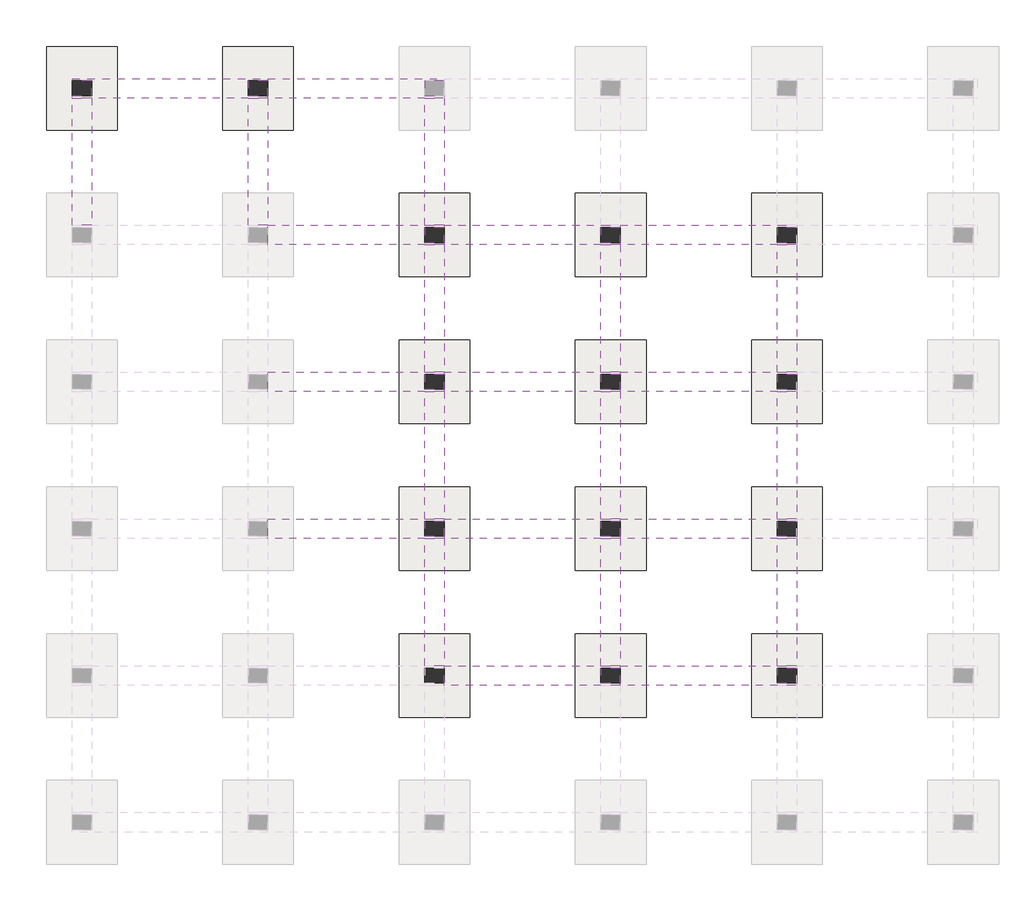
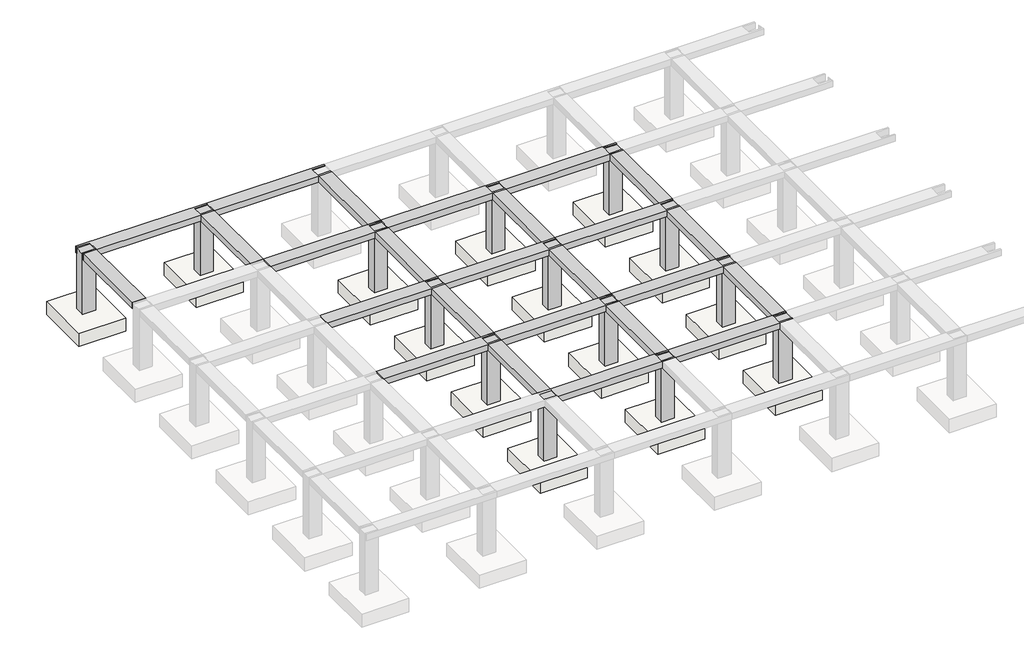
# One storey, part 2 of 3: 25 beams, 14 columns, 14 slabs.
"""IFC4 building model written with IfcOpenShell, lengths in millimetres."""

from ifc_helpers import new_model, si_unit, frame, origin, place, context, project, spatial, polyline, outline, extrude, faceted_brep, element, save

model = new_model("IFC4")

# Units and contexts
model_context = context("Model", 3, world=origin())
ifc_project = project(units=[si_unit("LENGTHUNIT", "METRE", prefix="MILLI")], contexts=[model_context])

# Site, building, storey
site = spatial("IfcSite", under=ifc_project)
building = spatial("IfcBuilding", under=site)
storey = spatial("IfcBuildingStorey", under=building, Elevation=-2999.978125)

# Beams
placement = place(None, origin())
element("IfcBeam", 1, ObjectType="Concrete-Rectangular Beam : 2' x2'", at=placement, inside=storey, context=model_context, shape_type="Brep", body=[
    faceted_brep([(-5646.474232, 1680.7831222, 48.021875), (-6256.074232, 1680.7831222, 48.021875), (-11132.874232, 1680.7831222, 48.021875), (-11132.874232, 1604.5831222, 48.021875), (-11132.874232, 1147.3831222, 48.021875), (-11132.874232, 1071.1831222, 48.021875), (-6256.074232, 1071.1831222, 48.021875), (-5646.474232, 1071.1831222, 48.021875), (-5646.474232, 1147.3831222, 48.021875), (-6256.074232, 1147.3831222, 48.021875), (-6256.074232, 1604.5831222, 48.021875), (-5646.474232, 1604.5831222, 48.021875), (-5646.474232, 1071.1831222, -256.778125), (-11132.874232, 1071.1831222, -256.778125), (-6256.074232, 1071.1831222, -256.778125), (-6256.074232, 1147.3831222, -256.778125), (-5646.474232, 1147.3831222, -256.778125), (-11132.874232, 1147.3831222, -256.778125), (-11132.874232, 1604.5831222, -256.778125), (-11132.874232, 1680.7831222, -256.778125), (-6256.074232, 1680.7831222, -256.778125), (-5646.474232, 1680.7831222, -256.778125), (-5646.474232, 1604.5831222, -256.778125), (-6256.074232, 1604.5831222, -256.778125)], [[[0, 1, 2, 3, 4, 5, 6, 7, 8, 9, 10, 11]], [[12, 7, 6, 5, 13, 14]], [[15, 16, 12, 14, 13, 17, 18, 19, 20, 21, 22, 23]], [[0, 21, 20, 19, 2, 1]], [[5, 4, 3, 2, 19, 18, 17, 13]], [[9, 8, 16, 15]], [[9, 15, 23, 10]], [[10, 23, 22, 11]], [[7, 12, 16, 8]], [[21, 0, 11, 22]]]),
])
element("IfcBeam", 2, ObjectType="Concrete-Rectangular Beam : 2' x2'", at=placement, inside=storey, context=model_context, shape_type="Brep", body=[
    faceted_brep([(-5646.474232, 1680.7831222, 48.021875), (-5646.474232, 1604.5831222, 48.021875), (-5646.474232, 1147.3831222, 48.021875), (-5646.474232, 1071.1831222, 48.021875), (-769.674232, 1071.1831222, 48.021875), (-160.074232, 1071.1831222, 48.021875), (-160.074232, 1147.3831222, 48.021875), (-769.674232, 1147.3831222, 48.021875), (-769.674232, 1604.5831222, 48.021875), (-160.074232, 1604.5831222, 48.021875), (-160.074232, 1680.7831222, 48.021875), (-769.674232, 1680.7831222, 48.021875), (-5646.474232, 1071.1831222, -256.778125), (-769.674232, 1071.1831222, -256.778125), (-160.074232, 1071.1831222, -256.778125), (-769.674232, 1147.3831222, -256.778125), (-160.074232, 1147.3831222, -256.778125), (-5646.474232, 1147.3831222, -256.778125), (-5646.474232, 1604.5831222, -256.778125), (-5646.474232, 1680.7831222, -256.778125), (-769.674232, 1680.7831222, -256.778125), (-160.074232, 1680.7831222, -256.778125), (-160.074232, 1604.5831222, -256.778125), (-769.674232, 1604.5831222, -256.778125)], [[[0, 1, 2, 3, 4, 5, 6, 7, 8, 9, 10, 11]], [[3, 12, 13, 14, 5, 4]], [[15, 16, 14, 13, 12, 17, 18, 19, 20, 21, 22, 23]], [[10, 21, 20, 19, 0, 11]], [[3, 2, 1, 0, 19, 18, 17, 12]], [[7, 6, 16, 15]], [[7, 15, 23, 8]], [[8, 23, 22, 9]], [[5, 14, 16, 6]], [[21, 10, 9, 22]]]),
])
element("IfcBeam", 3, ObjectType="Concrete-Rectangular Beam : 2' x2'", at=placement, inside=storey, context=model_context, shape_type="Brep", body=[
    faceted_brep([(-16619.274232, 6252.7831222, 48.021875), (-16619.274232, 6176.5831222, 48.021875), (-16619.274232, 5719.3831222, 48.021875), (-16619.274232, 5643.1831222, 48.021875), (-11742.474232, 5643.1831222, 48.021875), (-11132.874232, 5643.1831222, 48.021875), (-11132.874232, 5719.3831222, 48.021875), (-11742.474232, 5719.3831222, 48.021875), (-11742.474232, 6176.5831222, 48.021875), (-11132.874232, 6176.5831222, 48.021875), (-11132.874232, 6252.7831222, 48.021875), (-11742.474232, 6252.7831222, 48.021875), (-16619.274232, 5643.1831222, -256.778125), (-11742.474232, 5643.1831222, -256.778125), (-11132.874232, 5643.1831222, -256.778125), (-11742.474232, 5719.3831222, -256.778125), (-11132.874232, 5719.3831222, -256.778125), (-16619.274232, 5719.3831222, -256.778125), (-16619.274232, 6176.5831222, -256.778125), (-16619.274232, 6252.7831222, -256.778125), (-11742.474232, 6252.7831222, -256.778125), (-11132.874232, 6252.7831222, -256.778125), (-11132.874232, 6176.5831222, -256.778125), (-11742.474232, 6176.5831222, -256.778125)], [[[0, 1, 2, 3, 4, 5, 6, 7, 8, 9, 10, 11]], [[3, 12, 13, 14, 5, 4]], [[15, 16, 14, 13, 12, 17, 18, 19, 20, 21, 22, 23]], [[10, 21, 20, 19, 0, 11]], [[3, 2, 1, 0, 19, 18, 17, 12]], [[7, 6, 16, 15]], [[7, 15, 23, 8]], [[8, 23, 22, 9]], [[5, 14, 16, 6]], [[21, 10, 9, 22]]]),
])
element("IfcBeam", 4, ObjectType="Concrete-Rectangular Beam : 2' x2'", at=placement, inside=storey, context=model_context, shape_type="Brep", body=[
    faceted_brep([(-5646.474232, 6252.7831222, 48.021875), (-6256.074232, 6252.7831222, 48.021875), (-11132.874232, 6252.7831222, 48.021875), (-11132.874232, 6176.5831222, 48.021875), (-11132.874232, 5719.3831222, 48.021875), (-11132.874232, 5643.1831222, 48.021875), (-6256.074232, 5643.1831222, 48.021875), (-5646.474232, 5643.1831222, 48.021875), (-5646.474232, 5719.3831222, 48.021875), (-6256.074232, 5719.3831222, 48.021875), (-6256.074232, 6176.5831222, 48.021875), (-5646.474232, 6176.5831222, 48.021875), (-5646.474232, 5643.1831222, -256.778125), (-11132.874232, 5643.1831222, -256.778125), (-6256.074232, 5643.1831222, -256.778125), (-6256.074232, 5719.3831222, -256.778125), (-5646.474232, 5719.3831222, -256.778125), (-11132.874232, 5719.3831222, -256.778125), (-11132.874232, 6176.5831222, -256.778125), (-11132.874232, 6252.7831222, -256.778125), (-6256.074232, 6252.7831222, -256.778125), (-5646.474232, 6252.7831222, -256.778125), (-5646.474232, 6176.5831222, -256.778125), (-6256.074232, 6176.5831222, -256.778125)], [[[0, 1, 2, 3, 4, 5, 6, 7, 8, 9, 10, 11]], [[12, 7, 6, 5, 13, 14]], [[15, 16, 12, 14, 13, 17, 18, 19, 20, 21, 22, 23]], [[0, 21, 20, 19, 2, 1]], [[5, 4, 3, 2, 19, 18, 17, 13]], [[9, 8, 16, 15]], [[9, 15, 23, 10]], [[10, 23, 22, 11]], [[7, 12, 16, 8]], [[21, 0, 11, 22]]]),
])
element("IfcBeam", 5, ObjectType="Concrete-Rectangular Beam : 2' x2'", at=placement, inside=storey, context=model_context, shape_type="Brep", body=[
    faceted_brep([(-5646.474232, 6252.7831222, 48.021875), (-5646.474232, 6176.5831222, 48.021875), (-5646.474232, 5719.3831222, 48.021875), (-5646.474232, 5643.1831222, 48.021875), (-769.674232, 5643.1831222, 48.021875), (-160.074232, 5643.1831222, 48.021875), (-160.074232, 5719.3831222, 48.021875), (-769.674232, 5719.3831222, 48.021875), (-769.674232, 6176.5831222, 48.021875), (-160.074232, 6176.5831222, 48.021875), (-160.074232, 6252.7831222, 48.021875), (-769.674232, 6252.7831222, 48.021875), (-5646.474232, 5643.1831222, -256.778125), (-769.674232, 5643.1831222, -256.778125), (-160.074232, 5643.1831222, -256.778125), (-769.674232, 5719.3831222, -256.778125), (-160.074232, 5719.3831222, -256.778125), (-5646.474232, 5719.3831222, -256.778125), (-5646.474232, 6176.5831222, -256.778125), (-5646.474232, 6252.7831222, -256.778125), (-769.674232, 6252.7831222, -256.778125), (-160.074232, 6252.7831222, -256.778125), (-160.074232, 6176.5831222, -256.778125), (-769.674232, 6176.5831222, -256.778125)], [[[0, 1, 2, 3, 4, 5, 6, 7, 8, 9, 10, 11]], [[3, 12, 13, 14, 5, 4]], [[15, 16, 14, 13, 12, 17, 18, 19, 20, 21, 22, 23]], [[10, 21, 20, 19, 0, 11]], [[3, 2, 1, 0, 19, 18, 17, 12]], [[7, 6, 16, 15]], [[7, 15, 23, 8]], [[8, 23, 22, 9]], [[5, 14, 16, 6]], [[21, 10, 9, 22]]]),
])
element("IfcBeam", 6, ObjectType="Concrete-Rectangular Beam : 2' x2'", at=placement, inside=storey, context=model_context, shape_type="Brep", body=[
    faceted_brep([(-16619.274232, 10824.7831222, 48.021875), (-16619.274232, 10748.5831222, 48.021875), (-16619.274232, 10291.3831222, 48.021875), (-16619.274232, 10215.1831222, 48.021875), (-11742.474232, 10215.1831222, 48.021875), (-11132.874232, 10215.1831222, 48.021875), (-11132.874232, 10291.3831222, 48.021875), (-11742.474232, 10291.3831222, 48.021875), (-11742.474232, 10748.5831222, 48.021875), (-11132.874232, 10748.5831222, 48.021875), (-11132.874232, 10824.7831222, 48.021875), (-11742.474232, 10824.7831222, 48.021875), (-16619.274232, 10215.1831222, -256.778125), (-11742.474232, 10215.1831222, -256.778125), (-11132.874232, 10215.1831222, -256.778125), (-11742.474232, 10291.3831222, -256.778125), (-11132.874232, 10291.3831222, -256.778125), (-16619.274232, 10291.3831222, -256.778125), (-16619.274232, 10748.5831222, -256.778125), (-16619.274232, 10824.7831222, -256.778125), (-11742.474232, 10824.7831222, -256.778125), (-11132.874232, 10824.7831222, -256.778125), (-11132.874232, 10748.5831222, -256.778125), (-11742.474232, 10748.5831222, -256.778125)], [[[0, 1, 2, 3, 4, 5, 6, 7, 8, 9, 10, 11]], [[3, 12, 13, 14, 5, 4]], [[15, 16, 14, 13, 12, 17, 18, 19, 20, 21, 22, 23]], [[10, 21, 20, 19, 0, 11]], [[3, 2, 1, 0, 19, 18, 17, 12]], [[7, 6, 16, 15]], [[7, 15, 23, 8]], [[8, 23, 22, 9]], [[5, 14, 16, 6]], [[21, 10, 9, 22]]]),
])
element("IfcBeam", 7, ObjectType="Concrete-Rectangular Beam : 2' x2'", at=placement, inside=storey, context=model_context, shape_type="Brep", body=[
    faceted_brep([(-11132.874232, 10824.7831222, 48.021875), (-11132.874232, 10748.5831222, 48.021875), (-11132.874232, 10291.3831222, 48.021875), (-11132.874232, 10215.1831222, 48.021875), (-6256.074232, 10215.1831222, 48.021875), (-5646.474232, 10215.1831222, 48.021875), (-5646.474232, 10291.3831222, 48.021875), (-6256.074232, 10291.3831222, 48.021875), (-6256.074232, 10748.5831222, 48.021875), (-5646.474232, 10748.5831222, 48.021875), (-5646.474232, 10824.7831222, 48.021875), (-6256.074232, 10824.7831222, 48.021875), (-11132.874232, 10215.1831222, -256.778125), (-6256.074232, 10215.1831222, -256.778125), (-5646.474232, 10215.1831222, -256.778125), (-6256.074232, 10291.3831222, -256.778125), (-5646.474232, 10291.3831222, -256.778125), (-11132.874232, 10291.3831222, -256.778125), (-11132.874232, 10748.5831222, -256.778125), (-11132.874232, 10824.7831222, -256.778125), (-6256.074232, 10824.7831222, -256.778125), (-5646.474232, 10824.7831222, -256.778125), (-5646.474232, 10748.5831222, -256.778125), (-6256.074232, 10748.5831222, -256.778125)], [[[0, 1, 2, 3, 4, 5, 6, 7, 8, 9, 10, 11]], [[3, 12, 13, 14, 5, 4]], [[15, 16, 14, 13, 12, 17, 18, 19, 20, 21, 22, 23]], [[10, 21, 20, 19, 0, 11]], [[3, 2, 1, 0, 19, 18, 17, 12]], [[7, 6, 16, 15]], [[7, 15, 23, 8]], [[8, 23, 22, 9]], [[5, 14, 16, 6]], [[21, 10, 9, 22]]]),
])
element("IfcBeam", 8, ObjectType="Concrete-Rectangular Beam : 2' x2'", at=placement, inside=storey, context=model_context, shape_type="Brep", body=[
    faceted_brep([(-5646.474232, 10824.7831222, 48.021875), (-5646.474232, 10748.5831222, 48.021875), (-5646.474232, 10291.3831222, 48.021875), (-5646.474232, 10215.1831222, 48.021875), (-769.674232, 10215.1831222, 48.021875), (-160.074232, 10215.1831222, 48.021875), (-160.074232, 10291.3831222, 48.021875), (-769.674232, 10291.3831222, 48.021875), (-769.674232, 10748.5831222, 48.021875), (-160.074232, 10748.5831222, 48.021875), (-160.074232, 10824.7831222, 48.021875), (-769.674232, 10824.7831222, 48.021875), (-5646.474232, 10215.1831222, -256.778125), (-769.674232, 10215.1831222, -256.778125), (-160.074232, 10215.1831222, -256.778125), (-769.674232, 10291.3831222, -256.778125), (-160.074232, 10291.3831222, -256.778125), (-5646.474232, 10291.3831222, -256.778125), (-5646.474232, 10748.5831222, -256.778125), (-5646.474232, 10824.7831222, -256.778125), (-769.674232, 10824.7831222, -256.778125), (-160.074232, 10824.7831222, -256.778125), (-160.074232, 10748.5831222, -256.778125), (-769.674232, 10748.5831222, -256.778125)], [[[0, 1, 2, 3, 4, 5, 6, 7, 8, 9, 10, 11]], [[3, 12, 13, 14, 5, 4]], [[15, 16, 14, 13, 12, 17, 18, 19, 20, 21, 22, 23]], [[10, 21, 20, 19, 0, 11]], [[3, 2, 1, 0, 19, 18, 17, 12]], [[7, 6, 16, 15]], [[7, 15, 23, 8]], [[8, 23, 22, 9]], [[5, 14, 16, 6]], [[21, 10, 9, 22]]]),
])
element("IfcBeam", 9, ObjectType="Concrete-Rectangular Beam : 2' x2'", at=placement, inside=storey, context=model_context, shape_type="Brep", body=[
    faceted_brep([(-16619.274232, 15396.7831222, 48.021875), (-16619.274232, 15320.5831222, 48.021875), (-16619.274232, 14863.3831222, 48.021875), (-16619.274232, 14787.1831222, 48.021875), (-11742.474232, 14787.1831222, 48.021875), (-11132.874232, 14787.1831222, 48.021875), (-11132.874232, 14863.3831222, 48.021875), (-11742.474232, 14863.3831222, 48.021875), (-11742.474232, 15320.5831222, 48.021875), (-11132.874232, 15320.5831222, 48.021875), (-11132.874232, 15396.7831222, 48.021875), (-11742.474232, 15396.7831222, 48.021875), (-16619.274232, 14787.1831222, -256.778125), (-11742.474232, 14787.1831222, -256.778125), (-11132.874232, 14787.1831222, -256.778125), (-11742.474232, 14863.3831222, -256.778125), (-11132.874232, 14863.3831222, -256.778125), (-16619.274232, 14863.3831222, -256.778125), (-16619.274232, 15320.5831222, -256.778125), (-16619.274232, 15396.7831222, -256.778125), (-11742.474232, 15396.7831222, -256.778125), (-11132.874232, 15396.7831222, -256.778125), (-11132.874232, 15320.5831222, -256.778125), (-11742.474232, 15320.5831222, -256.778125)], [[[0, 1, 2, 3, 4, 5, 6, 7, 8, 9, 10, 11]], [[3, 12, 13, 14, 5, 4]], [[15, 16, 14, 13, 12, 17, 18, 19, 20, 21, 22, 23]], [[10, 21, 20, 19, 0, 11]], [[3, 2, 1, 0, 19, 18, 17, 12]], [[7, 6, 16, 15]], [[7, 15, 23, 8]], [[8, 23, 22, 9]], [[5, 14, 16, 6]], [[21, 10, 9, 22]]]),
])
element("IfcBeam", 10, ObjectType="Concrete-Rectangular Beam : 2' x2'", at=placement, inside=storey, context=model_context, shape_type="Brep", body=[
    faceted_brep([(-11132.874232, 15396.7831222, 48.021875), (-11132.874232, 15320.5831222, 48.021875), (-11132.874232, 14863.3831222, 48.021875), (-11132.874232, 14787.1831222, 48.021875), (-6256.074232, 14787.1831222, 48.021875), (-5646.474232, 14787.1831222, 48.021875), (-5646.474232, 14863.3831222, 48.021875), (-6256.074232, 14863.3831222, 48.021875), (-6256.074232, 15320.5831222, 48.021875), (-5646.474232, 15320.5831222, 48.021875), (-5646.474232, 15396.7831222, 48.021875), (-6256.074232, 15396.7831222, 48.021875), (-11132.874232, 14787.1831222, -256.778125), (-6256.074232, 14787.1831222, -256.778125), (-5646.474232, 14787.1831222, -256.778125), (-6256.074232, 14863.3831222, -256.778125), (-5646.474232, 14863.3831222, -256.778125), (-11132.874232, 14863.3831222, -256.778125), (-11132.874232, 15320.5831222, -256.778125), (-11132.874232, 15396.7831222, -256.778125), (-6256.074232, 15396.7831222, -256.778125), (-5646.474232, 15396.7831222, -256.778125), (-5646.474232, 15320.5831222, -256.778125), (-6256.074232, 15320.5831222, -256.778125)], [[[0, 1, 2, 3, 4, 5, 6, 7, 8, 9, 10, 11]], [[3, 12, 13, 14, 5, 4]], [[15, 16, 14, 13, 12, 17, 18, 19, 20, 21, 22, 23]], [[10, 21, 20, 19, 0, 11]], [[3, 2, 1, 0, 19, 18, 17, 12]], [[7, 6, 16, 15]], [[7, 15, 23, 8]], [[8, 23, 22, 9]], [[5, 14, 16, 6]], [[21, 10, 9, 22]]]),
])
element("IfcBeam", 11, ObjectType="Concrete-Rectangular Beam : 2' x2'", at=placement, inside=storey, context=model_context, shape_type="Brep", body=[
    faceted_brep([(-5646.474232, 15396.7831222, 48.021875), (-5646.474232, 15320.5831222, 48.021875), (-5646.474232, 14863.3831222, 48.021875), (-5646.474232, 14787.1831222, 48.021875), (-769.674232, 14787.1831222, 48.021875), (-160.074232, 14787.1831222, 48.021875), (-160.074232, 14863.3831222, 48.021875), (-769.674232, 14863.3831222, 48.021875), (-769.674232, 15320.5831222, 48.021875), (-160.074232, 15320.5831222, 48.021875), (-160.074232, 15396.7831222, 48.021875), (-769.674232, 15396.7831222, 48.021875), (-5646.474232, 14787.1831222, -256.778125), (-769.674232, 14787.1831222, -256.778125), (-160.074232, 14787.1831222, -256.778125), (-769.674232, 14863.3831222, -256.778125), (-160.074232, 14863.3831222, -256.778125), (-5646.474232, 14863.3831222, -256.778125), (-5646.474232, 15320.5831222, -256.778125), (-5646.474232, 15396.7831222, -256.778125), (-769.674232, 15396.7831222, -256.778125), (-160.074232, 15396.7831222, -256.778125), (-160.074232, 15320.5831222, -256.778125), (-769.674232, 15320.5831222, -256.778125)], [[[0, 1, 2, 3, 4, 5, 6, 7, 8, 9, 10, 11]], [[3, 12, 13, 14, 5, 4]], [[15, 16, 14, 13, 12, 17, 18, 19, 20, 21, 22, 23]], [[10, 21, 20, 19, 0, 11]], [[3, 2, 1, 0, 19, 18, 17, 12]], [[7, 6, 16, 15]], [[7, 15, 23, 8]], [[8, 23, 22, 9]], [[5, 14, 16, 6]], [[21, 10, 9, 22]]]),
])
element("IfcBeam", 12, ObjectType="Concrete-Rectangular Beam : 2' x2'", at=placement, inside=storey, context=model_context, shape_type="Brep", body=[
    faceted_brep([(-16619.274232, 19968.7831222, 48.021875), (-22715.274232, 19968.7831222, 48.021875), (-22715.274232, 19892.5831222, 48.021875), (-22105.674232, 19892.5831222, 48.021875), (-22105.674232, 19435.3831222, 48.021875), (-22715.274232, 19435.3831222, 48.021875), (-22715.274232, 19359.1831222, 48.021875), (-22105.674232, 19359.1831222, 48.021875), (-17228.874232, 19359.1831222, 48.021875), (-16619.274232, 19359.1831222, 48.021875), (-16619.274232, 19435.3831222, 48.021875), (-17228.874232, 19435.3831222, 48.021875), (-17228.874232, 19892.5831222, 48.021875), (-16619.274232, 19892.5831222, 48.021875), (-22715.274232, 19359.1831222, -256.778125), (-22105.674232, 19359.1831222, -256.778125), (-17228.874232, 19359.1831222, -256.778125), (-16619.274232, 19359.1831222, -256.778125), (-17228.874232, 19435.3831222, -256.778125), (-16619.274232, 19435.3831222, -256.778125), (-22715.274232, 19435.3831222, -256.778125), (-22105.674232, 19435.3831222, -256.778125), (-22105.674232, 19892.5831222, -256.778125), (-22715.274232, 19892.5831222, -256.778125), (-22715.274232, 19968.7831222, -256.778125), (-16619.274232, 19968.7831222, -256.778125), (-16619.274232, 19892.5831222, -256.778125), (-17228.874232, 19892.5831222, -256.778125)], [[[0, 1, 2, 3, 4, 5, 6, 7, 8, 9, 10, 11, 12, 13]], [[6, 14, 15, 16, 17, 9, 8, 7]], [[18, 19, 17, 16, 15, 14, 20, 21, 22, 23, 24, 25, 26, 27]], [[24, 1, 0, 25]], [[22, 21, 4, 3]], [[21, 20, 5, 4]], [[23, 22, 3, 2]], [[11, 10, 19, 18]], [[11, 18, 27, 12]], [[12, 27, 26, 13]], [[14, 6, 5, 20]], [[9, 17, 19, 10]], [[1, 24, 23, 2]], [[25, 0, 13, 26]]]),
])
element("IfcBeam", 13, ObjectType="Concrete-Rectangular Beam : 2' x2'", at=placement, inside=storey, context=model_context, shape_type="Brep", body=[
    faceted_brep([(-11132.874232, 19968.7831222, 48.021875), (-16619.274232, 19968.7831222, 48.021875), (-16619.274232, 19892.5831222, 48.021875), (-16619.274232, 19435.3831222, 48.021875), (-16619.274232, 19359.1831222, 48.021875), (-11742.474232, 19359.1831222, 48.021875), (-11132.874232, 19359.1831222, 48.021875), (-11132.874232, 19435.3831222, 48.021875), (-11742.474232, 19435.3831222, 48.021875), (-11742.474232, 19892.5831222, 48.021875), (-11132.874232, 19892.5831222, 48.021875), (-11132.874232, 19359.1831222, -256.778125), (-16619.274232, 19359.1831222, -256.778125), (-11742.474232, 19359.1831222, -256.778125), (-11742.474232, 19435.3831222, -256.778125), (-11132.874232, 19435.3831222, -256.778125), (-16619.274232, 19435.3831222, -256.778125), (-16619.274232, 19892.5831222, -256.778125), (-16619.274232, 19968.7831222, -256.778125), (-11132.874232, 19968.7831222, -256.778125), (-11132.874232, 19892.5831222, -256.778125), (-11742.474232, 19892.5831222, -256.778125)], [[[0, 1, 2, 3, 4, 5, 6, 7, 8, 9, 10]], [[11, 6, 5, 4, 12, 13]], [[14, 15, 11, 13, 12, 16, 17, 18, 19, 20, 21]], [[0, 19, 18, 1]], [[4, 3, 2, 1, 18, 17, 16, 12]], [[8, 7, 15, 14]], [[8, 14, 21, 9]], [[9, 21, 20, 10]], [[6, 11, 15, 7]], [[19, 0, 10, 20]]]),
])
element("IfcBeam", 14, ObjectType="Concrete-Rectangular Beam : 2' x2'", at=placement, inside=storey, context=model_context, shape_type="SweptSolid", body=[
    extrude(outline(polyline([(-22105.674232, 15396.7831222), (-22715.274232, 15396.7831222), (-22715.274232, 19359.1831222), (-22105.674232, 19359.1831222), (-22105.674232, 15396.7831222)])), frame((0.0, 0.0, -256.778125), z_axis=(0.0, 0.0, 1.0), x_axis=(1.0, 0.0, 0.0)), (0.0, 0.0, 1.0), 304.8),
])
element("IfcBeam", 15, ObjectType="Concrete-Rectangular Beam : 2' x2'", at=placement, inside=storey, context=model_context, shape_type="SweptSolid", body=[
    extrude(outline(polyline([(-16619.274232, 15396.7831222), (-17228.874232, 15396.7831222), (-17228.874232, 19359.1831222), (-16619.274232, 19359.1831222), (-16619.274232, 15396.7831222)])), frame((0.0, 0.0, -256.778125), z_axis=(0.0, 0.0, 1.0), x_axis=(1.0, 0.0, 0.0)), (0.0, 0.0, 1.0), 304.8),
])
element("IfcBeam", 16, ObjectType="Concrete-Rectangular Beam : 2' x2'", at=placement, inside=storey, context=model_context, shape_type="SweptSolid", body=[
    extrude(outline(polyline([(-11132.874232, 1680.7831222), (-11742.474232, 1680.7831222), (-11742.474232, 5643.1831222), (-11132.874232, 5643.1831222), (-11132.874232, 1680.7831222)])), frame((0.0, 0.0, -256.778125), z_axis=(0.0, 0.0, 1.0), x_axis=(1.0, 0.0, 0.0)), (0.0, 0.0, 1.0), 304.8),
])
element("IfcBeam", 17, ObjectType="Concrete-Rectangular Beam : 2' x2'", at=placement, inside=storey, context=model_context, shape_type="SweptSolid", body=[
    extrude(outline(polyline([(-11132.874232, 6252.7831222), (-11742.474232, 6252.7831222), (-11742.474232, 10215.1831222), (-11132.874232, 10215.1831222), (-11132.874232, 6252.7831222)])), frame((0.0, 0.0, -256.778125), z_axis=(0.0, 0.0, 1.0), x_axis=(1.0, 0.0, 0.0)), (0.0, 0.0, 1.0), 304.8),
])
element("IfcBeam", 18, ObjectType="Concrete-Rectangular Beam : 2' x2'", at=placement, inside=storey, context=model_context, shape_type="SweptSolid", body=[
    extrude(outline(polyline([(-11132.874232, 10824.7831222), (-11742.474232, 10824.7831222), (-11742.474232, 14787.1831222), (-11132.874232, 14787.1831222), (-11132.874232, 10824.7831222)])), frame((0.0, 0.0, -256.778125), z_axis=(0.0, 0.0, 1.0), x_axis=(1.0, 0.0, 0.0)), (0.0, 0.0, 1.0), 304.8),
])
element("IfcBeam", 19, ObjectType="Concrete-Rectangular Beam : 2' x2'", at=placement, inside=storey, context=model_context, shape_type="SweptSolid", body=[
    extrude(outline(polyline([(-11132.874232, 15396.7831222), (-11742.474232, 15396.7831222), (-11742.474232, 19359.1831222), (-11132.874232, 19359.1831222), (-11132.874232, 15396.7831222)])), frame((0.0, 0.0, -256.778125), z_axis=(0.0, 0.0, 1.0), x_axis=(1.0, 0.0, 0.0)), (0.0, 0.0, 1.0), 304.8),
])
element("IfcBeam", 20, ObjectType="Concrete-Rectangular Beam : 2' x2'", at=placement, inside=storey, context=model_context, shape_type="SweptSolid", body=[
    extrude(outline(polyline([(-5646.474232, 1680.7831222), (-6256.074232, 1680.7831222), (-6256.074232, 5643.1831222), (-5646.474232, 5643.1831222), (-5646.474232, 1680.7831222)])), frame((0.0, 0.0, -256.778125), z_axis=(0.0, 0.0, 1.0), x_axis=(1.0, 0.0, 0.0)), (0.0, 0.0, 1.0), 304.8),
])
element("IfcBeam", 21, ObjectType="Concrete-Rectangular Beam : 2' x2'", at=placement, inside=storey, context=model_context, shape_type="SweptSolid", body=[
    extrude(outline(polyline([(-5646.474232, 6252.7831222), (-6256.074232, 6252.7831222), (-6256.074232, 10215.1831222), (-5646.474232, 10215.1831222), (-5646.474232, 6252.7831222)])), frame((0.0, 0.0, -256.778125), z_axis=(0.0, 0.0, 1.0), x_axis=(1.0, 0.0, 0.0)), (0.0, 0.0, 1.0), 304.8),
])
element("IfcBeam", 22, ObjectType="Concrete-Rectangular Beam : 2' x2'", at=placement, inside=storey, context=model_context, shape_type="SweptSolid", body=[
    extrude(outline(polyline([(-5646.474232, 10824.7831222), (-6256.074232, 10824.7831222), (-6256.074232, 14787.1831222), (-5646.474232, 14787.1831222), (-5646.474232, 10824.7831222)])), frame((0.0, 0.0, -256.778125), z_axis=(0.0, 0.0, 1.0), x_axis=(1.0, 0.0, 0.0)), (0.0, 0.0, 1.0), 304.8),
])
element("IfcBeam", 23, ObjectType="Concrete-Rectangular Beam : 2' x2'", at=placement, inside=storey, context=model_context, shape_type="SweptSolid", body=[
    extrude(outline(polyline([(-769.674232, 5643.1831222), (-160.074232, 5643.1831222), (-160.074232, 1680.7831222), (-769.674232, 1680.7831222), (-769.674232, 5643.1831222)])), frame((0.0, 0.0, -256.778125), z_axis=(0.0, 0.0, 1.0), x_axis=(1.0, 0.0, 0.0)), (0.0, 0.0, 1.0), 304.8),
])
element("IfcBeam", 24, ObjectType="Concrete-Rectangular Beam : 2' x2'", at=placement, inside=storey, context=model_context, shape_type="SweptSolid", body=[
    extrude(outline(polyline([(-160.074232, 6252.7831222), (-769.674232, 6252.7831222), (-769.674232, 10215.1831222), (-160.074232, 10215.1831222), (-160.074232, 6252.7831222)])), frame((0.0, 0.0, -256.778125), z_axis=(0.0, 0.0, 1.0), x_axis=(1.0, 0.0, 0.0)), (0.0, 0.0, 1.0), 304.8),
])
element("IfcBeam", 25, ObjectType="Concrete-Rectangular Beam : 2' x2'", at=placement, inside=storey, context=model_context, shape_type="SweptSolid", body=[
    extrude(outline(polyline([(-769.674232, 14787.1831222), (-160.074232, 14787.1831222), (-160.074232, 10824.7831222), (-769.674232, 10824.7831222), (-769.674232, 14787.1831222)])), frame((0.0, 0.0, -256.778125), z_axis=(0.0, 0.0, 1.0), x_axis=(1.0, 0.0, 0.0)), (0.0, 0.0, 1.0), 304.8),
])

# Columns
element("IfcColumn", 26, ObjectType="Concrete-Rectangular-Column : 12 x 18", at=placement, inside=storey, context=model_context, shape_type="SweptSolid", body=[
    extrude(outline(polyline([(-11132.874232, 1604.5831222), (-11132.874232, 1147.3831222), (-11742.474232, 1147.3831222), (-11742.474232, 1604.5831222), (-11132.874232, 1604.5831222)])), frame((0.0, 0.0, -2999.978125), z_axis=(0.0, 0.0, 1.0), x_axis=(1.0, 0.0, 0.0)), (0.0, 0.0, 1.0), 2999.978125),
])
element("IfcColumn", 27, ObjectType="Concrete-Rectangular-Column : 12 x 18", at=placement, inside=storey, context=model_context, shape_type="SweptSolid", body=[
    extrude(outline(polyline([(-5646.474232, 1604.5831222), (-5646.474232, 1147.3831222), (-6256.074232, 1147.3831222), (-6256.074232, 1604.5831222), (-5646.474232, 1604.5831222)])), frame((0.0, 0.0, -2999.978125), z_axis=(0.0, 0.0, 1.0), x_axis=(1.0, 0.0, 0.0)), (0.0, 0.0, 1.0), 2999.978125),
])
element("IfcColumn", 28, ObjectType="Concrete-Rectangular-Column : 12 x 18", at=placement, inside=storey, context=model_context, shape_type="SweptSolid", body=[
    extrude(outline(polyline([(-160.074232, 1604.5831222), (-160.074232, 1147.3831222), (-769.674232, 1147.3831222), (-769.674232, 1604.5831222), (-160.074232, 1604.5831222)])), frame((0.0, 0.0, -2999.978125), z_axis=(0.0, 0.0, 1.0), x_axis=(1.0, 0.0, 0.0)), (0.0, 0.0, 1.0), 2999.978125),
])
element("IfcColumn", 29, ObjectType="Concrete-Rectangular-Column : 12 x 18", at=placement, inside=storey, context=model_context, shape_type="SweptSolid", body=[
    extrude(outline(polyline([(-11132.874232, 6176.5831222), (-11132.874232, 5719.3831222), (-11742.474232, 5719.3831222), (-11742.474232, 6176.5831222), (-11132.874232, 6176.5831222)])), frame((0.0, 0.0, -2999.978125), z_axis=(0.0, 0.0, 1.0), x_axis=(1.0, 0.0, 0.0)), (0.0, 0.0, 1.0), 2999.978125),
])
element("IfcColumn", 30, ObjectType="Concrete-Rectangular-Column : 12 x 18", at=placement, inside=storey, context=model_context, shape_type="SweptSolid", body=[
    extrude(outline(polyline([(-5646.474232, 6176.5831222), (-5646.474232, 5719.3831222), (-6256.074232, 5719.3831222), (-6256.074232, 6176.5831222), (-5646.474232, 6176.5831222)])), frame((0.0, 0.0, -2999.978125), z_axis=(0.0, 0.0, 1.0), x_axis=(1.0, 0.0, 0.0)), (0.0, 0.0, 1.0), 2999.978125),
])
element("IfcColumn", 31, ObjectType="Concrete-Rectangular-Column : 12 x 18", at=placement, inside=storey, context=model_context, shape_type="SweptSolid", body=[
    extrude(outline(polyline([(-160.074232, 6176.5831222), (-160.074232, 5719.3831222), (-769.674232, 5719.3831222), (-769.674232, 6176.5831222), (-160.074232, 6176.5831222)])), frame((0.0, 0.0, -2999.978125), z_axis=(0.0, 0.0, 1.0), x_axis=(1.0, 0.0, 0.0)), (0.0, 0.0, 1.0), 2999.978125),
])
element("IfcColumn", 32, ObjectType="Concrete-Rectangular-Column : 12 x 18", at=placement, inside=storey, context=model_context, shape_type="SweptSolid", body=[
    extrude(outline(polyline([(-11132.874232, 10748.5831222), (-11132.874232, 10291.3831222), (-11742.474232, 10291.3831222), (-11742.474232, 10748.5831222), (-11132.874232, 10748.5831222)])), frame((0.0, 0.0, -2999.978125), z_axis=(0.0, 0.0, 1.0), x_axis=(1.0, 0.0, 0.0)), (0.0, 0.0, 1.0), 2999.978125),
])
element("IfcColumn", 33, ObjectType="Concrete-Rectangular-Column : 12 x 18", at=placement, inside=storey, context=model_context, shape_type="SweptSolid", body=[
    extrude(outline(polyline([(-5646.474232, 10748.5831222), (-5646.474232, 10291.3831222), (-6256.074232, 10291.3831222), (-6256.074232, 10748.5831222), (-5646.474232, 10748.5831222)])), frame((0.0, 0.0, -2999.978125), z_axis=(0.0, 0.0, 1.0), x_axis=(1.0, 0.0, 0.0)), (0.0, 0.0, 1.0), 2999.978125),
])
element("IfcColumn", 34, ObjectType="Concrete-Rectangular-Column : 12 x 18", at=placement, inside=storey, context=model_context, shape_type="SweptSolid", body=[
    extrude(outline(polyline([(-160.074232, 10748.5831222), (-160.074232, 10291.3831222), (-769.674232, 10291.3831222), (-769.674232, 10748.5831222), (-160.074232, 10748.5831222)])), frame((0.0, 0.0, -2999.978125), z_axis=(0.0, 0.0, 1.0), x_axis=(1.0, 0.0, 0.0)), (0.0, 0.0, 1.0), 2999.978125),
])
element("IfcColumn", 35, ObjectType="Concrete-Rectangular-Column : 12 x 18", at=placement, inside=storey, context=model_context, shape_type="SweptSolid", body=[
    extrude(outline(polyline([(-11132.874232, 15320.5831222), (-11132.874232, 14863.3831222), (-11742.474232, 14863.3831222), (-11742.474232, 15320.5831222), (-11132.874232, 15320.5831222)])), frame((0.0, 0.0, -2999.978125), z_axis=(0.0, 0.0, 1.0), x_axis=(1.0, 0.0, 0.0)), (0.0, 0.0, 1.0), 2999.978125),
])
element("IfcColumn", 36, ObjectType="Concrete-Rectangular-Column : 12 x 18", at=placement, inside=storey, context=model_context, shape_type="SweptSolid", body=[
    extrude(outline(polyline([(-5646.474232, 15320.5831222), (-5646.474232, 14863.3831222), (-6256.074232, 14863.3831222), (-6256.074232, 15320.5831222), (-5646.474232, 15320.5831222)])), frame((0.0, 0.0, -2999.978125), z_axis=(0.0, 0.0, 1.0), x_axis=(1.0, 0.0, 0.0)), (0.0, 0.0, 1.0), 2999.978125),
])
element("IfcColumn", 37, ObjectType="Concrete-Rectangular-Column : 12 x 18", at=placement, inside=storey, context=model_context, shape_type="SweptSolid", body=[
    extrude(outline(polyline([(-160.074232, 15320.5831222), (-160.074232, 14863.3831222), (-769.674232, 14863.3831222), (-769.674232, 15320.5831222), (-160.074232, 15320.5831222)])), frame((0.0, 0.0, -2999.978125), z_axis=(0.0, 0.0, 1.0), x_axis=(1.0, 0.0, 0.0)), (0.0, 0.0, 1.0), 2999.978125),
])
element("IfcColumn", 38, ObjectType="Concrete-Rectangular-Column : 12 x 18", at=placement, inside=storey, context=model_context, shape_type="SweptSolid", body=[
    extrude(outline(polyline([(-22105.674232, 19892.5831222), (-22105.674232, 19435.3831222), (-22715.274232, 19435.3831222), (-22715.274232, 19892.5831222), (-22105.674232, 19892.5831222)])), frame((0.0, 0.0, -2999.978125), z_axis=(0.0, 0.0, 1.0), x_axis=(1.0, 0.0, 0.0)), (0.0, 0.0, 1.0), 2999.978125),
])
element("IfcColumn", 39, ObjectType="Concrete-Rectangular-Column : 12 x 18", at=placement, inside=storey, context=model_context, shape_type="SweptSolid", body=[
    extrude(outline(polyline([(-16619.274232, 19892.5831222), (-16619.274232, 19435.3831222), (-17228.874232, 19435.3831222), (-17228.874232, 19892.5831222), (-16619.274232, 19892.5831222)])), frame((0.0, 0.0, -2999.978125), z_axis=(0.0, 0.0, 1.0), x_axis=(1.0, 0.0, 0.0)), (0.0, 0.0, 1.0), 2999.978125),
])

# Slabs
element("IfcSlab", 40, ObjectType="Footing-Rectangular : 650 X 2200X2600", at=placement, inside=storey, context=model_context, shape_type="SweptSolid", body=[
    extrude(outline(polyline([(-10337.6855602, 2675.9967941), (-10337.6855602, 75.9694503), (-12537.6629039, 75.9694503), (-12537.6629039, 2675.9967941), (-10337.6855602, 2675.9967941)])), frame((0.0, 0.0, -3649.9601562), z_axis=(0.0, 0.0, 1.0), x_axis=(1.0, 0.0, 0.0)), (0.0, 0.0, 1.0), 649.9820313),
])
element("IfcSlab", 41, ObjectType="Footing-Rectangular : 650 X 2200X2600", at=placement, inside=storey, context=model_context, shape_type="SweptSolid", body=[
    extrude(outline(polyline([(-4851.2855602, 2675.9967941), (-4851.2855602, 75.9694503), (-7051.2629039, 75.9694503), (-7051.2629039, 2675.9967941), (-4851.2855602, 2675.9967941)])), frame((0.0, 0.0, -3649.9601562), z_axis=(0.0, 0.0, 1.0), x_axis=(1.0, 0.0, 0.0)), (0.0, 0.0, 1.0), 649.9820313),
])
element("IfcSlab", 42, ObjectType="Footing-Rectangular : 650 X 2200X2600", at=placement, inside=storey, context=model_context, shape_type="SweptSolid", body=[
    extrude(outline(polyline([(635.1144398, 2675.9967941), (635.1144398, 75.9694503), (-1564.8629039, 75.9694503), (-1564.8629039, 2675.9967941), (635.1144398, 2675.9967941)])), frame((0.0, 0.0, -3649.9601562), z_axis=(0.0, 0.0, 1.0), x_axis=(1.0, 0.0, 0.0)), (0.0, 0.0, 1.0), 649.9820313),
])
element("IfcSlab", 43, ObjectType="Footing-Rectangular : 650 X 2200X2600", at=placement, inside=storey, context=model_context, shape_type="SweptSolid", body=[
    extrude(outline(polyline([(-10337.6855602, 7247.9967941), (-10337.6855602, 4647.9694503), (-12537.6629039, 4647.9694503), (-12537.6629039, 7247.9967941), (-10337.6855602, 7247.9967941)])), frame((0.0, 0.0, -3649.9601562), z_axis=(0.0, 0.0, 1.0), x_axis=(1.0, 0.0, 0.0)), (0.0, 0.0, 1.0), 649.9820313),
])
element("IfcSlab", 44, ObjectType="Footing-Rectangular : 650 X 2200X2600", at=placement, inside=storey, context=model_context, shape_type="SweptSolid", body=[
    extrude(outline(polyline([(-4851.2855602, 7247.9967941), (-4851.2855602, 4647.9694503), (-7051.2629039, 4647.9694503), (-7051.2629039, 7247.9967941), (-4851.2855602, 7247.9967941)])), frame((0.0, 0.0, -3649.9601562), z_axis=(0.0, 0.0, 1.0), x_axis=(1.0, 0.0, 0.0)), (0.0, 0.0, 1.0), 649.9820313),
])
element("IfcSlab", 45, ObjectType="Footing-Rectangular : 650 X 2200X2600", at=placement, inside=storey, context=model_context, shape_type="SweptSolid", body=[
    extrude(outline(polyline([(635.1144398, 7247.9967941), (635.1144398, 4647.9694503), (-1564.8629039, 4647.9694503), (-1564.8629039, 7247.9967941), (635.1144398, 7247.9967941)])), frame((0.0, 0.0, -3649.9601562), z_axis=(0.0, 0.0, 1.0), x_axis=(1.0, 0.0, 0.0)), (0.0, 0.0, 1.0), 649.9820313),
])
element("IfcSlab", 46, ObjectType="Footing-Rectangular : 650 X 2200X2600", at=placement, inside=storey, context=model_context, shape_type="SweptSolid", body=[
    extrude(outline(polyline([(-10337.6855602, 11819.9967941), (-10337.6855602, 9219.9694503), (-12537.6629039, 9219.9694503), (-12537.6629039, 11819.9967941), (-10337.6855602, 11819.9967941)])), frame((0.0, 0.0, -3649.9601562), z_axis=(0.0, 0.0, 1.0), x_axis=(1.0, 0.0, 0.0)), (0.0, 0.0, 1.0), 649.9820313),
])
element("IfcSlab", 47, ObjectType="Footing-Rectangular : 650 X 2200X2600", at=placement, inside=storey, context=model_context, shape_type="SweptSolid", body=[
    extrude(outline(polyline([(-4851.2855602, 11819.9967941), (-4851.2855602, 9219.9694503), (-7051.2629039, 9219.9694503), (-7051.2629039, 11819.9967941), (-4851.2855602, 11819.9967941)])), frame((0.0, 0.0, -3649.9601562), z_axis=(0.0, 0.0, 1.0), x_axis=(1.0, 0.0, 0.0)), (0.0, 0.0, 1.0), 649.9820313),
])
element("IfcSlab", 48, ObjectType="Footing-Rectangular : 650 X 2200X2600", at=placement, inside=storey, context=model_context, shape_type="SweptSolid", body=[
    extrude(outline(polyline([(635.1144398, 11819.9967941), (635.1144398, 9219.9694503), (-1564.8629039, 9219.9694503), (-1564.8629039, 11819.9967941), (635.1144398, 11819.9967941)])), frame((0.0, 0.0, -3649.9601562), z_axis=(0.0, 0.0, 1.0), x_axis=(1.0, 0.0, 0.0)), (0.0, 0.0, 1.0), 649.9820313),
])
element("IfcSlab", 49, ObjectType="Footing-Rectangular : 650 X 2200X2600", at=placement, inside=storey, context=model_context, shape_type="SweptSolid", body=[
    extrude(outline(polyline([(-10337.6855602, 16391.9967941), (-10337.6855602, 13791.9694503), (-12537.6629039, 13791.9694503), (-12537.6629039, 16391.9967941), (-10337.6855602, 16391.9967941)])), frame((0.0, 0.0, -3649.9601562), z_axis=(0.0, 0.0, 1.0), x_axis=(1.0, 0.0, 0.0)), (0.0, 0.0, 1.0), 649.9820313),
])
element("IfcSlab", 50, ObjectType="Footing-Rectangular : 650 X 2200X2600", at=placement, inside=storey, context=model_context, shape_type="SweptSolid", body=[
    extrude(outline(polyline([(-4851.2855602, 16391.9967941), (-4851.2855602, 13791.9694503), (-7051.2629039, 13791.9694503), (-7051.2629039, 16391.9967941), (-4851.2855602, 16391.9967941)])), frame((0.0, 0.0, -3649.9601562), z_axis=(0.0, 0.0, 1.0), x_axis=(1.0, 0.0, 0.0)), (0.0, 0.0, 1.0), 649.9820313),
])
element("IfcSlab", 51, ObjectType="Footing-Rectangular : 650 X 2200X2600", at=placement, inside=storey, context=model_context, shape_type="SweptSolid", body=[
    extrude(outline(polyline([(635.1144398, 16391.9967941), (635.1144398, 13791.9694503), (-1564.8629039, 13791.9694503), (-1564.8629039, 16391.9967941), (635.1144398, 16391.9967941)])), frame((0.0, 0.0, -3649.9601562), z_axis=(0.0, 0.0, 1.0), x_axis=(1.0, 0.0, 0.0)), (0.0, 0.0, 1.0), 649.9820313),
])
element("IfcSlab", 52, ObjectType="Footing-Rectangular : 650 X 2200X2600", at=placement, inside=storey, context=model_context, shape_type="SweptSolid", body=[
    extrude(outline(polyline([(-21310.4855602, 20963.9967941), (-21310.4855602, 18363.9694503), (-23510.4629039, 18363.9694503), (-23510.4629039, 20963.9967941), (-21310.4855602, 20963.9967941)])), frame((0.0, 0.0, -3649.9601562), z_axis=(0.0, 0.0, 1.0), x_axis=(1.0, 0.0, 0.0)), (0.0, 0.0, 1.0), 649.9820313),
])
element("IfcSlab", 53, ObjectType="Footing-Rectangular : 650 X 2200X2600", at=placement, inside=storey, context=model_context, shape_type="SweptSolid", body=[
    extrude(outline(polyline([(-15824.0855602, 20963.9967941), (-15824.0855602, 18363.9694503), (-18024.0629039, 18363.9694503), (-18024.0629039, 20963.9967941), (-15824.0855602, 20963.9967941)])), frame((0.0, 0.0, -3649.9601562), z_axis=(0.0, 0.0, 1.0), x_axis=(1.0, 0.0, 0.0)), (0.0, 0.0, 1.0), 649.9820313),
])

save(model, "model.ifc")

# Revit data of these elements
# Type "Concrete-Rectangular Beam : 2' x2'"
#   Assembly Code = "B10"
#   Length [instance default] = 5' - 0"
#   b = 2' - 0"
#   h = 1' - 0"
#   Structural Material [instance default] = Concrete, Cast-in-Place gray
# Type "Concrete-Rectangular-Column : 12 x 18"
#   Assembly Code = "B10"
#   b = 2' - 0"
#   h = 1' - 6"
#   Structural Material [instance default] = Concrete, Cast-in-Place gray
# Type "Footing-Rectangular : 650 X 2200X2600"
#   Assembly Code = "A1010100"
#   Width = 7' - 2 157/256"
#   Length = 8' - 6 93/256"
#   Foundation Thickness = 2' - 1 151/256"
#   Structural Material [instance default] = Concrete, Cast-in-Place gray
# Elements 1, 2, 3, 4, 5, 6, 7, 8, 9, 10, 11, 12, 13, 14, 15, 16, 17, 18, 19, 20, 21, 22, 23, 24, 25 (IfcBeam, "Concrete-Rectangular Beam : 2' x2'")
#   Structural Material = Concrete, Precast (2)
#   Phase Created = New Construction
#   Materials on its faces: "Concrete, Precast (2)"
# Elements 26, 27, 28, 29, 30, 31, 32, 33, 34, 35, 36, 37, 38, 39 (IfcColumn, "Concrete-Rectangular-Column : 12 x 18")
#   Phase Created = New Construction
#   Materials on its faces: "Concrete, Cast-in-Place gray"
# Elements 40, 41, 42, 43, 44, 45, 46, 47, 48, 49, 50, 51, 53 (IfcSlab, "Footing-Rectangular : 650 X 2200X2600")
#   Structural Material = Concrete, Cast-in-Place gray
#   Phase Created = New Construction
#   Materials on its faces: "Concrete, Cast-in-Place gray"
# Element 52 (IfcSlab, "Footing-Rectangular : 650 X 2200X2600")
#   Structural Material = Concrete, Precast
#   Phase Created = New Construction
#   Materials on its faces: "Concrete, Precast"
# Materials
#   "Concrete, Cast-in-Place gray": class "Concrete", colour RGB 192 192 192, transparency 0, Description = "Cast-in-place concrete", Cost = 0
#   "Concrete, Precast (2)": class "Concrete", colour RGB 198 187 187, transparency 0, Description = "Precast concrete", Cost = 0
#   "Concrete, Precast": class "Concrete", colour RGB 198 187 187, transparency 0, Description = "Precast concrete", Cost = 0
